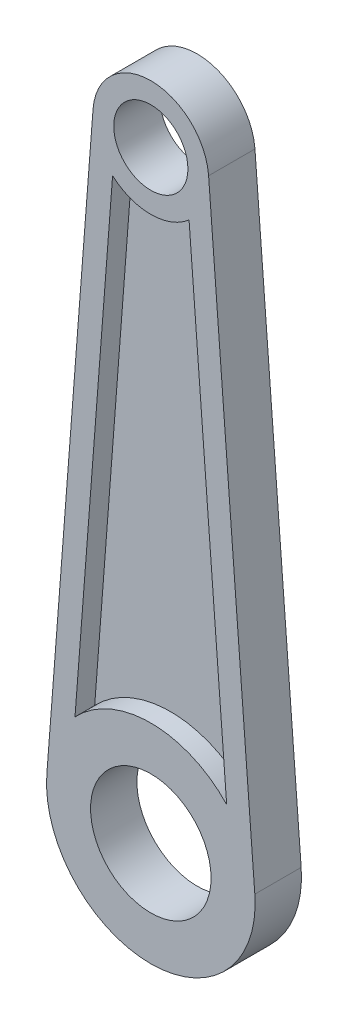
ISO-10303-21;
HEADER;
FILE_DESCRIPTION(('STEP AP214'),'2;1');
FILE_NAME('part.step','',(''),(''),'','','');
FILE_SCHEMA(('AUTOMOTIVE_DESIGN { 1 0 10303 214 1 1 1 1 }'));
ENDSEC;
DATA;
#1=APPLICATION_CONTEXT('core data for automotive mechanical design processes');
#2=APPLICATION_PROTOCOL_DEFINITION('international standard','automotive_design',2000,#1);
#3=PRODUCT_CONTEXT('',#1,'mechanical');
#4=PRODUCT('Part','Part','',(#3));
#5=PRODUCT_RELATED_PRODUCT_CATEGORY('part','',(#4));
#6=PRODUCT_DEFINITION_FORMATION('','',#4);
#7=PRODUCT_DEFINITION_CONTEXT('part definition',#1,'design');
#8=PRODUCT_DEFINITION('design','',#6,#7);
#9=PRODUCT_DEFINITION_SHAPE('','',#8);
#10=(LENGTH_UNIT() NAMED_UNIT(*) SI_UNIT(.MILLI.,.METRE.));
#11=(NAMED_UNIT(*) PLANE_ANGLE_UNIT() SI_UNIT($,.RADIAN.));
#12=(NAMED_UNIT(*) SI_UNIT($,.STERADIAN.) SOLID_ANGLE_UNIT());
#13=UNCERTAINTY_MEASURE_WITH_UNIT(LENGTH_MEASURE(1.E-05),#10,'distance_accuracy_value','');
#14=(GEOMETRIC_REPRESENTATION_CONTEXT(3) GLOBAL_UNCERTAINTY_ASSIGNED_CONTEXT((#13)) GLOBAL_UNIT_ASSIGNED_CONTEXT((#10,
#11,#12)) REPRESENTATION_CONTEXT('',''));
#15=CARTESIAN_POINT('',(0.,0.,0.));
#16=DIRECTION('',(0.,0.,1.));
#17=DIRECTION('',(1.,0.,0.));
#18=AXIS2_PLACEMENT_3D('',#15,#16,#17);
#19=CARTESIAN_POINT('',(0.,-65.,5.));
#20=DIRECTION('',(0.,0.,-1.));
#21=DIRECTION('',(-1.,0.,0.));
#22=AXIS2_PLACEMENT_3D('',#19,#20,#21);
#23=CYLINDRICAL_SURFACE('',#22,22.5);
#24=DIRECTION('',(0.,0.,-1.));
#25=VECTOR('',#24,1.);
#26=CARTESIAN_POINT('',(-16.3602914477342,-49.5536132462897,5.));
#27=LINE('',#26,#25);
#28=CARTESIAN_POINT('',(-16.3602914477342,-49.5536132462897,-0.75));
#29=VERTEX_POINT('',#28);
#30=CARTESIAN_POINT('',(-16.3602914477342,-49.5536132462897,-5.));
#31=VERTEX_POINT('',#30);
#32=EDGE_CURVE('E145',#29,#31,#27,.T.);
#33=ORIENTED_EDGE('',*,*,#32,.F.);
#34=CARTESIAN_POINT('',(0.,-65.,-0.75));
#35=DIRECTION('',(0.,0.,1.));
#36=DIRECTION('',(1.,0.,0.));
#37=AXIS2_PLACEMENT_3D('',#34,#35,#36);
#38=CIRCLE('',#37,22.5);
#39=CARTESIAN_POINT('',(16.3602914477342,-49.5536132462897,-0.75));
#40=VERTEX_POINT('',#39);
#41=EDGE_CURVE('E165',#40,#29,#38,.T.);
#42=ORIENTED_EDGE('',*,*,#41,.F.);
#43=DIRECTION('',(0.,0.,-1.));
#44=VECTOR('',#43,1.);
#45=CARTESIAN_POINT('',(16.3602914477342,-49.5536132462897,5.));
#46=LINE('',#45,#44);
#47=CARTESIAN_POINT('',(16.3602914477342,-49.5536132462897,-5.));
#48=VERTEX_POINT('',#47);
#49=EDGE_CURVE('E192',#40,#48,#46,.T.);
#50=ORIENTED_EDGE('',*,*,#49,.T.);
#51=CARTESIAN_POINT('',(0.,-65.,-5.));
#52=DIRECTION('',(0.,0.,-1.));
#53=DIRECTION('',(1.,0.,0.));
#54=AXIS2_PLACEMENT_3D('',#51,#52,#53);
#55=CIRCLE('',#54,22.5);
#56=EDGE_CURVE('E152',#31,#48,#55,.T.);
#57=ORIENTED_EDGE('',*,*,#56,.F.);
#58=EDGE_LOOP('',(#33,#42,#50,#57));
#59=FACE_BOUND('',#58,.T.);
#60=ADVANCED_FACE('F43',(#59),#23,.T.);
#61=CARTESIAN_POINT('',(8.24700849816291,55.6065527716802,5.));
#62=DIRECTION('',(-0.997037030524286,-0.076923076923077,0.));
#63=DIRECTION('',(0.076923076923077,-0.997037030524286,0.));
#64=AXIS2_PLACEMENT_3D('',#61,#62,#63);
#65=PLANE('',#64);
#66=ORIENTED_EDGE('',*,*,#49,.F.);
#67=DIRECTION('',(0.076923076923077,-0.997037030524286,0.));
#68=VECTOR('',#67,1.);
#69=CARTESIAN_POINT('',(12.4629628815536,0.961538461538461,-0.75));
#70=LINE('',#69,#68);
#71=CARTESIAN_POINT('',(8.2470084981629,55.6065527716802,-0.75));
#72=VERTEX_POINT('',#71);
#73=EDGE_CURVE('E163',#72,#40,#70,.T.);
#74=ORIENTED_EDGE('',*,*,#73,.F.);
#75=DIRECTION('',(0.,0.,-1.));
#76=VECTOR('',#75,1.);
#77=CARTESIAN_POINT('',(8.24700849816291,55.6065527716802,5.));
#78=LINE('',#77,#76);
#79=CARTESIAN_POINT('',(8.24700849816291,55.6065527716802,-5.));
#80=VERTEX_POINT('',#79);
#81=EDGE_CURVE('E187',#72,#80,#78,.T.);
#82=ORIENTED_EDGE('',*,*,#81,.T.);
#83=DIRECTION('',(-0.076923076923077,0.997037030524286,0.));
#84=VECTOR('',#83,1.);
#85=CARTESIAN_POINT('',(8.24700849816291,55.6065527716802,-5.));
#86=LINE('',#85,#84);
#87=EDGE_CURVE('E160',#48,#80,#86,.T.);
#88=ORIENTED_EDGE('',*,*,#87,.F.);
#89=EDGE_LOOP('',(#66,#74,#82,#88));
#90=FACE_BOUND('',#89,.T.);
#91=ADVANCED_FACE('F259',(#90),#65,.T.);
#92=CARTESIAN_POINT('',(0.,65.,5.));
#93=DIRECTION('',(0.,0.,-1.));
#94=DIRECTION('',(-1.,0.,0.));
#95=AXIS2_PLACEMENT_3D('',#92,#93,#94);
#96=CYLINDRICAL_SURFACE('',#95,12.5);
#97=ORIENTED_EDGE('',*,*,#81,.F.);
#98=CARTESIAN_POINT('',(0.,65.,-0.75));
#99=DIRECTION('',(0.,0.,1.));
#100=DIRECTION('',(1.,0.,0.));
#101=AXIS2_PLACEMENT_3D('',#98,#99,#100);
#102=CIRCLE('',#101,12.5);
#103=CARTESIAN_POINT('',(-8.24700849816293,55.6065527716802,-0.75));
#104=VERTEX_POINT('',#103);
#105=EDGE_CURVE('E167',#104,#72,#102,.T.);
#106=ORIENTED_EDGE('',*,*,#105,.F.);
#107=DIRECTION('',(0.,0.,-1.));
#108=VECTOR('',#107,1.);
#109=CARTESIAN_POINT('',(-8.24700849816293,55.6065527716802,5.));
#110=LINE('',#109,#108);
#111=CARTESIAN_POINT('',(-8.24700849816293,55.6065527716802,-5.));
#112=VERTEX_POINT('',#111);
#113=EDGE_CURVE('E141',#104,#112,#110,.T.);
#114=ORIENTED_EDGE('',*,*,#113,.T.);
#115=CARTESIAN_POINT('',(0.,65.,-5.));
#116=DIRECTION('',(0.,0.,-1.));
#117=DIRECTION('',(1.,0.,0.));
#118=AXIS2_PLACEMENT_3D('',#115,#116,#117);
#119=CIRCLE('',#118,12.5);
#120=EDGE_CURVE('E182',#80,#112,#119,.T.);
#121=ORIENTED_EDGE('',*,*,#120,.F.);
#122=EDGE_LOOP('',(#97,#106,#114,#121));
#123=FACE_BOUND('',#122,.T.);
#124=ADVANCED_FACE('F266',(#123),#96,.T.);
#125=CARTESIAN_POINT('',(-8.24700849816293,55.6065527716802,5.));
#126=DIRECTION('',(0.997037030524286,-0.0769230769230768,0.));
#127=DIRECTION('',(0.0769230769230768,0.997037030524286,0.));
#128=AXIS2_PLACEMENT_3D('',#125,#126,#127);
#129=PLANE('',#128);
#130=ORIENTED_EDGE('',*,*,#113,.F.);
#131=DIRECTION('',(-0.0769230769230768,-0.997037030524286,0.));
#132=VECTOR('',#131,1.);
#133=CARTESIAN_POINT('',(-12.4629628815536,0.961538461538461,-0.75));
#134=LINE('',#133,#132);
#135=EDGE_CURVE('E151',#104,#29,#134,.T.);
#136=ORIENTED_EDGE('',*,*,#135,.T.);
#137=ORIENTED_EDGE('',*,*,#32,.T.);
#138=DIRECTION('',(-0.0769230769230768,-0.997037030524286,0.));
#139=VECTOR('',#138,1.);
#140=CARTESIAN_POINT('',(-8.24700849816293,55.6065527716802,-5.));
#141=LINE('',#140,#139);
#142=EDGE_CURVE('E172',#112,#31,#141,.T.);
#143=ORIENTED_EDGE('',*,*,#142,.F.);
#144=EDGE_LOOP('',(#130,#136,#137,#143));
#145=FACE_BOUND('',#144,.T.);
#146=ADVANCED_FACE('F288',(#145),#129,.T.);
#147=CARTESIAN_POINT('',(0.,65.,5.));
#148=DIRECTION('',(0.,0.,1.));
#149=DIRECTION('',(1.,0.,0.));
#150=AXIS2_PLACEMENT_3D('',#147,#148,#149);
#151=PLANE('',#150);
#152=CARTESIAN_POINT('',(0.,65.,5.));
#153=DIRECTION('',(0.,0.,1.));
#154=DIRECTION('',(1.,0.,0.));
#155=AXIS2_PLACEMENT_3D('',#152,#153,#154);
#156=CIRCLE('',#155,8.00000000000001);
#157=CARTESIAN_POINT('',(7.99999999999999,65.,5.));
#158=VERTEX_POINT('',#157);
#159=EDGE_CURVE('E199',#158,#158,#156,.T.);
#160=ORIENTED_EDGE('',*,*,#159,.F.);
#161=EDGE_LOOP('',(#160));
#162=FACE_BOUND('',#161,.T.);
#163=CARTESIAN_POINT('',(0.,65.,5.));
#164=DIRECTION('',(0.,0.,1.));
#165=DIRECTION('',(1.,0.,0.));
#166=AXIS2_PLACEMENT_3D('',#163,#164,#165);
#167=CIRCLE('',#166,12.5);
#168=CARTESIAN_POINT('',(12.4629628815536,65.9615384615385,5.));
#169=VERTEX_POINT('',#168);
#170=CARTESIAN_POINT('',(-12.4629628815536,65.9615384615385,5.));
#171=VERTEX_POINT('',#170);
#172=EDGE_CURVE('E206',#169,#171,#167,.T.);
#173=ORIENTED_EDGE('',*,*,#172,.T.);
#174=DIRECTION('',(-0.0769230769230769,-0.997037030524286,0.));
#175=VECTOR('',#174,1.);
#176=CARTESIAN_POINT('',(-12.4629628815536,65.9615384615385,5.));
#177=LINE('',#176,#175);
#178=CARTESIAN_POINT('',(-22.4333331867964,-63.2692307692308,5.));
#179=VERTEX_POINT('',#178);
#180=EDGE_CURVE('E207',#171,#179,#177,.T.);
#181=ORIENTED_EDGE('',*,*,#180,.T.);
#182=CARTESIAN_POINT('',(0.,-65.,5.));
#183=DIRECTION('',(0.,0.,1.));
#184=DIRECTION('',(1.,0.,0.));
#185=AXIS2_PLACEMENT_3D('',#182,#183,#184);
#186=CIRCLE('',#185,22.5);
#187=CARTESIAN_POINT('',(22.4333331867964,-63.2692307692308,5.));
#188=VERTEX_POINT('',#187);
#189=EDGE_CURVE('E215',#179,#188,#186,.T.);
#190=ORIENTED_EDGE('',*,*,#189,.T.);
#191=DIRECTION('',(-0.0769230769230771,0.997037030524286,0.));
#192=VECTOR('',#191,1.);
#193=CARTESIAN_POINT('',(12.4629628815536,65.9615384615385,5.));
#194=LINE('',#193,#192);
#195=EDGE_CURVE('E212',#188,#169,#194,.T.);
#196=ORIENTED_EDGE('',*,*,#195,.T.);
#197=EDGE_LOOP('',(#173,#181,#190,#196));
#198=FACE_BOUND('',#197,.T.);
#199=CARTESIAN_POINT('',(0.,-65.,5.));
#200=DIRECTION('',(0.,0.,1.));
#201=DIRECTION('',(1.,0.,0.));
#202=AXIS2_PLACEMENT_3D('',#199,#200,#201);
#203=CIRCLE('',#202,13.);
#204=CARTESIAN_POINT('',(13.,-65.,5.));
#205=VERTEX_POINT('',#204);
#206=EDGE_CURVE('E191',#205,#205,#203,.T.);
#207=ORIENTED_EDGE('',*,*,#206,.F.);
#208=EDGE_LOOP('',(#207));
#209=FACE_BOUND('',#208,.T.);
#210=DIRECTION('',(-0.076923076923077,0.997037030524286,0.));
#211=VECTOR('',#210,1.);
#212=CARTESIAN_POINT('',(8.24700849816291,55.6065527716802,5.));
#213=LINE('',#212,#211);
#214=CARTESIAN_POINT('',(16.3602914477342,-49.5536132462897,5.));
#215=VERTEX_POINT('',#214);
#216=CARTESIAN_POINT('',(8.24700849816291,55.6065527716802,5.));
#217=VERTEX_POINT('',#216);
#218=EDGE_CURVE('E175',#215,#217,#213,.T.);
#219=ORIENTED_EDGE('',*,*,#218,.F.);
#220=CARTESIAN_POINT('',(0.,-65.,5.));
#221=DIRECTION('',(0.,0.,-1.));
#222=DIRECTION('',(1.,0.,0.));
#223=AXIS2_PLACEMENT_3D('',#220,#221,#222);
#224=CIRCLE('',#223,22.5);
#225=CARTESIAN_POINT('',(-16.3602914477342,-49.5536132462897,5.));
#226=VERTEX_POINT('',#225);
#227=EDGE_CURVE('E168',#226,#215,#224,.T.);
#228=ORIENTED_EDGE('',*,*,#227,.F.);
#229=DIRECTION('',(-0.0769230769230768,-0.997037030524286,0.));
#230=VECTOR('',#229,1.);
#231=CARTESIAN_POINT('',(-8.24700849816293,55.6065527716802,5.));
#232=LINE('',#231,#230);
#233=CARTESIAN_POINT('',(-8.24700849816293,55.6065527716802,5.));
#234=VERTEX_POINT('',#233);
#235=EDGE_CURVE('E138',#234,#226,#232,.T.);
#236=ORIENTED_EDGE('',*,*,#235,.F.);
#237=CARTESIAN_POINT('',(0.,65.,5.));
#238=DIRECTION('',(0.,0.,-1.));
#239=DIRECTION('',(1.,0.,0.));
#240=AXIS2_PLACEMENT_3D('',#237,#238,#239);
#241=CIRCLE('',#240,12.5);
#242=EDGE_CURVE('E174',#217,#234,#241,.T.);
#243=ORIENTED_EDGE('',*,*,#242,.F.);
#244=EDGE_LOOP('',(#219,#228,#236,#243));
#245=FACE_BOUND('',#244,.T.);
#246=ADVANCED_FACE('F246',(#162,#198,#209,#245),#151,.T.);
#247=CARTESIAN_POINT('',(0.,65.,-5.));
#248=DIRECTION('',(0.,0.,1.));
#249=DIRECTION('',(1.,0.,0.));
#250=AXIS2_PLACEMENT_3D('',#247,#248,#249);
#251=PLANE('',#250);
#252=CARTESIAN_POINT('',(0.,-65.,-5.));
#253=DIRECTION('',(0.,0.,1.));
#254=DIRECTION('',(1.,0.,0.));
#255=AXIS2_PLACEMENT_3D('',#252,#253,#254);
#256=CIRCLE('',#255,13.);
#257=CARTESIAN_POINT('',(13.,-65.,-5.));
#258=VERTEX_POINT('',#257);
#259=EDGE_CURVE('E194',#258,#258,#256,.T.);
#260=ORIENTED_EDGE('',*,*,#259,.T.);
#261=EDGE_LOOP('',(#260));
#262=FACE_BOUND('',#261,.T.);
#263=CARTESIAN_POINT('',(0.,65.,-5.));
#264=DIRECTION('',(0.,0.,1.));
#265=DIRECTION('',(1.,0.,0.));
#266=AXIS2_PLACEMENT_3D('',#263,#264,#265);
#267=CIRCLE('',#266,8.00000000000001);
#268=CARTESIAN_POINT('',(7.99999999999999,65.,-5.));
#269=VERTEX_POINT('',#268);
#270=EDGE_CURVE('E197',#269,#269,#267,.T.);
#271=ORIENTED_EDGE('',*,*,#270,.T.);
#272=EDGE_LOOP('',(#271));
#273=FACE_BOUND('',#272,.T.);
#274=CARTESIAN_POINT('',(0.,65.,-5.));
#275=DIRECTION('',(0.,0.,1.));
#276=DIRECTION('',(1.,0.,0.));
#277=AXIS2_PLACEMENT_3D('',#274,#275,#276);
#278=CIRCLE('',#277,12.5);
#279=CARTESIAN_POINT('',(12.4629628815536,65.9615384615385,-5.));
#280=VERTEX_POINT('',#279);
#281=CARTESIAN_POINT('',(-12.4629628815536,65.9615384615385,-5.));
#282=VERTEX_POINT('',#281);
#283=EDGE_CURVE('E201',#280,#282,#278,.T.);
#284=ORIENTED_EDGE('',*,*,#283,.F.);
#285=DIRECTION('',(-0.0769230769230771,0.997037030524286,0.));
#286=VECTOR('',#285,1.);
#287=CARTESIAN_POINT('',(12.4629628815536,65.9615384615385,-5.));
#288=LINE('',#287,#286);
#289=CARTESIAN_POINT('',(22.4333331867964,-63.2692307692308,-5.));
#290=VERTEX_POINT('',#289);
#291=EDGE_CURVE('E209',#290,#280,#288,.T.);
#292=ORIENTED_EDGE('',*,*,#291,.F.);
#293=CARTESIAN_POINT('',(0.,-65.,-5.));
#294=DIRECTION('',(0.,0.,1.));
#295=DIRECTION('',(1.,0.,0.));
#296=AXIS2_PLACEMENT_3D('',#293,#294,#295);
#297=CIRCLE('',#296,22.5);
#298=CARTESIAN_POINT('',(-22.4333331867964,-63.2692307692308,-5.));
#299=VERTEX_POINT('',#298);
#300=EDGE_CURVE('E222',#299,#290,#297,.T.);
#301=ORIENTED_EDGE('',*,*,#300,.F.);
#302=DIRECTION('',(-0.0769230769230769,-0.997037030524286,0.));
#303=VECTOR('',#302,1.);
#304=CARTESIAN_POINT('',(-12.4629628815536,65.9615384615385,-5.));
#305=LINE('',#304,#303);
#306=EDGE_CURVE('E218',#282,#299,#305,.T.);
#307=ORIENTED_EDGE('',*,*,#306,.F.);
#308=EDGE_LOOP('',(#284,#292,#301,#307));
#309=FACE_BOUND('',#308,.T.);
#310=ORIENTED_EDGE('',*,*,#56,.T.);
#311=ORIENTED_EDGE('',*,*,#87,.T.);
#312=ORIENTED_EDGE('',*,*,#120,.T.);
#313=ORIENTED_EDGE('',*,*,#142,.T.);
#314=EDGE_LOOP('',(#310,#311,#312,#313));
#315=FACE_BOUND('',#314,.T.);
#316=ADVANCED_FACE('F239',(#262,#273,#309,#315),#251,.F.);
#317=CARTESIAN_POINT('',(0.,65.,5.));
#318=DIRECTION('',(0.,0.,-1.));
#319=DIRECTION('',(-1.,0.,0.));
#320=AXIS2_PLACEMENT_3D('',#317,#318,#319);
#321=CYLINDRICAL_SURFACE('',#320,12.5);
#322=ORIENTED_EDGE('',*,*,#283,.T.);
#323=DIRECTION('',(0.,0.,-1.));
#324=VECTOR('',#323,1.);
#325=CARTESIAN_POINT('',(-12.4629628815536,65.9615384615385,5.));
#326=LINE('',#325,#324);
#327=EDGE_CURVE('E11',#171,#282,#326,.T.);
#328=ORIENTED_EDGE('',*,*,#327,.F.);
#329=ORIENTED_EDGE('',*,*,#172,.F.);
#330=DIRECTION('',(0.,0.,-1.));
#331=VECTOR('',#330,1.);
#332=CARTESIAN_POINT('',(12.4629628815536,65.9615384615385,5.));
#333=LINE('',#332,#331);
#334=EDGE_CURVE('E216',#169,#280,#333,.T.);
#335=ORIENTED_EDGE('',*,*,#334,.T.);
#336=EDGE_LOOP('',(#322,#328,#329,#335));
#337=FACE_BOUND('',#336,.T.);
#338=ADVANCED_FACE('F44',(#337),#321,.T.);
#339=CARTESIAN_POINT('',(-12.4629628815536,65.9615384615385,5.));
#340=DIRECTION('',(0.997037030524286,-0.0769230769230769,0.));
#341=DIRECTION('',(0.0769230769230769,0.997037030524286,0.));
#342=AXIS2_PLACEMENT_3D('',#339,#340,#341);
#343=PLANE('',#342);
#344=ORIENTED_EDGE('',*,*,#306,.T.);
#345=DIRECTION('',(0.,0.,-1.));
#346=VECTOR('',#345,1.);
#347=CARTESIAN_POINT('',(-22.4333331867964,-63.2692307692308,5.));
#348=LINE('',#347,#346);
#349=EDGE_CURVE('E51',#179,#299,#348,.T.);
#350=ORIENTED_EDGE('',*,*,#349,.F.);
#351=ORIENTED_EDGE('',*,*,#180,.F.);
#352=ORIENTED_EDGE('',*,*,#327,.T.);
#353=EDGE_LOOP('',(#344,#350,#351,#352));
#354=FACE_BOUND('',#353,.T.);
#355=ADVANCED_FACE('F253',(#354),#343,.F.);
#356=CARTESIAN_POINT('',(0.,-65.,5.));
#357=DIRECTION('',(0.,0.,-1.));
#358=DIRECTION('',(-1.,0.,0.));
#359=AXIS2_PLACEMENT_3D('',#356,#357,#358);
#360=CYLINDRICAL_SURFACE('',#359,22.5);
#361=ORIENTED_EDGE('',*,*,#300,.T.);
#362=DIRECTION('',(0.,0.,-1.));
#363=VECTOR('',#362,1.);
#364=CARTESIAN_POINT('',(22.4333331867964,-63.2692307692308,5.));
#365=LINE('',#364,#363);
#366=EDGE_CURVE('E226',#188,#290,#365,.T.);
#367=ORIENTED_EDGE('',*,*,#366,.F.);
#368=ORIENTED_EDGE('',*,*,#189,.F.);
#369=ORIENTED_EDGE('',*,*,#349,.T.);
#370=EDGE_LOOP('',(#361,#367,#368,#369));
#371=FACE_BOUND('',#370,.T.);
#372=ADVANCED_FACE('F234',(#371),#360,.T.);
#373=CARTESIAN_POINT('',(12.4629628815536,65.9615384615385,5.));
#374=DIRECTION('',(-0.997037030524286,-0.0769230769230771,0.));
#375=DIRECTION('',(0.0769230769230771,-0.997037030524286,0.));
#376=AXIS2_PLACEMENT_3D('',#373,#374,#375);
#377=PLANE('',#376);
#378=ORIENTED_EDGE('',*,*,#291,.T.);
#379=ORIENTED_EDGE('',*,*,#334,.F.);
#380=ORIENTED_EDGE('',*,*,#195,.F.);
#381=ORIENTED_EDGE('',*,*,#366,.T.);
#382=EDGE_LOOP('',(#378,#379,#380,#381));
#383=FACE_BOUND('',#382,.T.);
#384=ADVANCED_FACE('F242',(#383),#377,.F.);
#385=CARTESIAN_POINT('',(0.,65.,5.));
#386=DIRECTION('',(0.,0.,-1.));
#387=DIRECTION('',(-1.,0.,0.));
#388=AXIS2_PLACEMENT_3D('',#385,#386,#387);
#389=CYLINDRICAL_SURFACE('',#388,8.00000000000001);
#390=ORIENTED_EDGE('',*,*,#159,.T.);
#391=EDGE_LOOP('',(#390));
#392=FACE_BOUND('',#391,.T.);
#393=ORIENTED_EDGE('',*,*,#270,.F.);
#394=EDGE_LOOP('',(#393));
#395=FACE_BOUND('',#394,.T.);
#396=ADVANCED_FACE('F276',(#392,#395),#389,.F.);
#397=CARTESIAN_POINT('',(0.,-65.,5.));
#398=DIRECTION('',(0.,0.,-1.));
#399=DIRECTION('',(-1.,0.,0.));
#400=AXIS2_PLACEMENT_3D('',#397,#398,#399);
#401=CYLINDRICAL_SURFACE('',#400,13.);
#402=ORIENTED_EDGE('',*,*,#206,.T.);
#403=EDGE_LOOP('',(#402));
#404=FACE_BOUND('',#403,.T.);
#405=ORIENTED_EDGE('',*,*,#259,.F.);
#406=EDGE_LOOP('',(#405));
#407=FACE_BOUND('',#406,.T.);
#408=ADVANCED_FACE('F272',(#404,#407),#401,.F.);
#409=CARTESIAN_POINT('',(0.,-65.,0.75));
#410=DIRECTION('',(0.,0.,1.));
#411=DIRECTION('',(1.,0.,0.));
#412=AXIS2_PLACEMENT_3D('',#409,#410,#411);
#413=CIRCLE('',#412,22.5);
#414=CARTESIAN_POINT('',(16.3602914477342,-49.5536132462897,0.75));
#415=VERTEX_POINT('',#414);
#416=CARTESIAN_POINT('',(-16.3602914477342,-49.5536132462897,0.75));
#417=VERTEX_POINT('',#416);
#418=EDGE_CURVE('E150',#415,#417,#413,.T.);
#419=ORIENTED_EDGE('',*,*,#418,.T.);
#420=EDGE_CURVE('E133',#226,#417,#27,.T.);
#421=ORIENTED_EDGE('',*,*,#420,.F.);
#422=ORIENTED_EDGE('',*,*,#227,.T.);
#423=EDGE_CURVE('E149',#215,#415,#46,.T.);
#424=ORIENTED_EDGE('',*,*,#423,.T.);
#425=EDGE_LOOP('',(#419,#421,#422,#424));
#426=FACE_BOUND('',#425,.T.);
#427=ADVANCED_FACE('F146',(#426),#23,.T.);
#428=DIRECTION('',(0.076923076923077,-0.997037030524286,0.));
#429=VECTOR('',#428,1.);
#430=CARTESIAN_POINT('',(12.4629628815536,0.961538461538461,0.75));
#431=LINE('',#430,#429);
#432=CARTESIAN_POINT('',(8.24700849816291,55.6065527716802,0.75));
#433=VERTEX_POINT('',#432);
#434=EDGE_CURVE('E59',#433,#415,#431,.T.);
#435=ORIENTED_EDGE('',*,*,#434,.T.);
#436=ORIENTED_EDGE('',*,*,#423,.F.);
#437=ORIENTED_EDGE('',*,*,#218,.T.);
#438=EDGE_CURVE('E188',#217,#433,#78,.T.);
#439=ORIENTED_EDGE('',*,*,#438,.T.);
#440=EDGE_LOOP('',(#435,#436,#437,#439));
#441=FACE_BOUND('',#440,.T.);
#442=ADVANCED_FACE('F267',(#441),#65,.T.);
#443=CARTESIAN_POINT('',(0.,65.,0.75));
#444=DIRECTION('',(0.,0.,1.));
#445=DIRECTION('',(1.,0.,0.));
#446=AXIS2_PLACEMENT_3D('',#443,#444,#445);
#447=CIRCLE('',#446,12.5);
#448=CARTESIAN_POINT('',(-8.24700849816293,55.6065527716802,0.75));
#449=VERTEX_POINT('',#448);
#450=EDGE_CURVE('E67',#449,#433,#447,.T.);
#451=ORIENTED_EDGE('',*,*,#450,.T.);
#452=ORIENTED_EDGE('',*,*,#438,.F.);
#453=ORIENTED_EDGE('',*,*,#242,.T.);
#454=EDGE_CURVE('E186',#234,#449,#110,.T.);
#455=ORIENTED_EDGE('',*,*,#454,.T.);
#456=EDGE_LOOP('',(#451,#452,#453,#455));
#457=FACE_BOUND('',#456,.T.);
#458=ADVANCED_FACE('F279',(#457),#96,.T.);
#459=DIRECTION('',(-0.0769230769230768,-0.997037030524286,0.));
#460=VECTOR('',#459,1.);
#461=CARTESIAN_POINT('',(-12.4629628815536,0.961538461538461,0.75));
#462=LINE('',#461,#460);
#463=EDGE_CURVE('E139',#449,#417,#462,.T.);
#464=ORIENTED_EDGE('',*,*,#463,.F.);
#465=ORIENTED_EDGE('',*,*,#454,.F.);
#466=ORIENTED_EDGE('',*,*,#235,.T.);
#467=ORIENTED_EDGE('',*,*,#420,.T.);
#468=EDGE_LOOP('',(#464,#465,#466,#467));
#469=FACE_BOUND('',#468,.T.);
#470=ADVANCED_FACE('F137',(#469),#129,.T.);
#471=CARTESIAN_POINT('',(0.,0.,-0.75));
#472=DIRECTION('',(0.,0.,1.));
#473=DIRECTION('',(1.,0.,0.));
#474=AXIS2_PLACEMENT_3D('',#471,#472,#473);
#475=PLANE('',#474);
#476=ORIENTED_EDGE('',*,*,#41,.T.);
#477=ORIENTED_EDGE('',*,*,#135,.F.);
#478=ORIENTED_EDGE('',*,*,#105,.T.);
#479=ORIENTED_EDGE('',*,*,#73,.T.);
#480=EDGE_LOOP('',(#476,#477,#478,#479));
#481=FACE_BOUND('',#480,.T.);
#482=ADVANCED_FACE('F340',(#481),#475,.F.);
#483=CARTESIAN_POINT('',(0.,0.,0.75));
#484=DIRECTION('',(0.,0.,1.));
#485=DIRECTION('',(1.,0.,0.));
#486=AXIS2_PLACEMENT_3D('',#483,#484,#485);
#487=PLANE('',#486);
#488=ORIENTED_EDGE('',*,*,#418,.F.);
#489=ORIENTED_EDGE('',*,*,#434,.F.);
#490=ORIENTED_EDGE('',*,*,#450,.F.);
#491=ORIENTED_EDGE('',*,*,#463,.T.);
#492=EDGE_LOOP('',(#488,#489,#490,#491));
#493=FACE_BOUND('',#492,.T.);
#494=ADVANCED_FACE('F153',(#493),#487,.T.);
#495=CLOSED_SHELL('',(#60,#91,#124,#146,#246,#316,#338,#355,#372,#384,#396,#408,#427,#442,#458,
#470,#482,#494));
#496=MANIFOLD_SOLID_BREP('B2',#495);
#497=ADVANCED_BREP_SHAPE_REPRESENTATION('',(#18,#496),#14);
#498=SHAPE_DEFINITION_REPRESENTATION(#9,#497);
ENDSEC;
END-ISO-10303-21;
